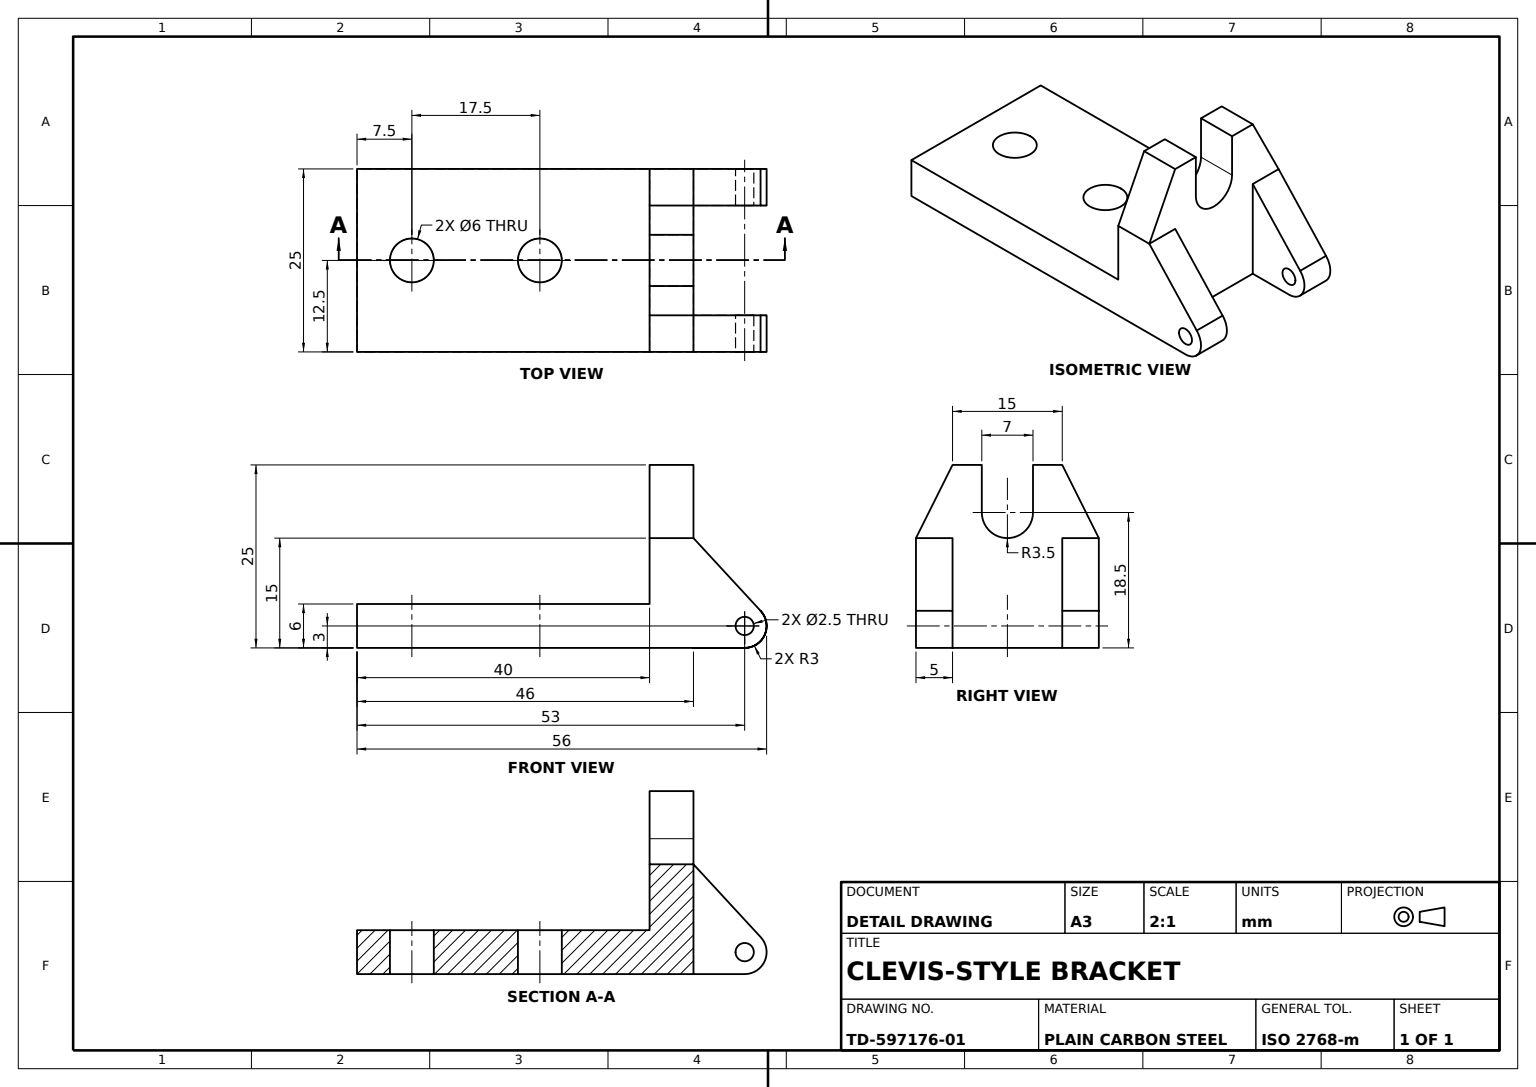
SolidWorks part; units mm, degrees
material "Plain Carbon Steel"
ref_plane "Front Plane" through (0, 0, 0) normal (0, 0, 1) x (1, 0, 0)
ref_plane "Top Plane" through (0, 0, 0) normal (0, 1, 0) x (1, 0, 0)
ref_plane "Right Plane" through (0, 0, 0) normal (1, 0, 0) x (0, 0, -1)
sketch "Base Profile Sketch" plane through (0, 0, 0) normal (0, 0, 1) x (1, 0, 0)
  line L0 (0, 0) -> (40, 0)
  line L1 (0, 0) -> (0, 6)
  line L2 (0, 6) -> (40, 6)
  line L3 (40, 6) -> (40, 0)
  dimension "D1" = 40
  dimension "D2" = 6
extrude "Base Body" add sketch "Base Profile Sketch" along normal blind 25
sketch "Upright Block Sketch" plane through (0, 0, 25) normal (0, 0, 1) x (1, 0, 0)
  line L0 (40, 0) -> (46, 0)
  line L1 (46, 0) -> (46, 15)
  line L2 (46, 15) -> (40, 15)
  line L3 (40, 15) -> (40, 0)
  line L4 (0, 6) -> (0, 0) construction
  line L5 (0, 0) -> (40, 0) construction
  dimension "D1" = 46
  dimension "D2" = 15
extrude "Upright Block" add sketch "Upright Block Sketch" against normal blind 25
sketch "Clevis Slot Profile Sketch" plane through (40, 0, 0) normal (-1, 0, 0) x (0, 0, 1)
  line L1 (25, 6) -> (0, 6) construction
  line L3 (9, 18.5) -> (9, 25)
  line L4 (16, 18.5) -> (16, 25)
  line L5 (16, 25) -> (20, 25)
  line L6 (20, 25) -> (25, 15)
  line L7 (9, 25) -> (5, 25)
  line L8 (5, 25) -> (0, 15)
  line L12 (0, 6) -> (25, 6)
  line L13 (25, 6) -> (25, 15)
  line L14 (25, 15) -> (0, 15)
  line L15 (0, 15) -> (0, 6)
  line L18 (25, 15) -> (0, 15)
  arc A0 (9, 18.5) -> (16, 18.5) centre (12.5, 18.5) ccw
  line M7 (25, 15) -> (0, 15)
  dimension "D1" = 0
  dimension "D2" = 3.5
  dimension "D3" = 5
  dimension "D4" = 19
extrude "Slotted Clevis Plate" add sketch "Clevis Slot Profile Sketch" against normal blind 6 contours A0 L6 L5 L4 M7 | A0 L3 L7 L8 L18
sketch "Lug 1 Sketch" plane through (0, 0, 25) normal (0, 0, 1) x (1, 0, 0)
  line L0 (46, 0) -> (53, 0)
  line L1 (0, 6) -> (0, 0) construction
  line L2 (46, 0) -> (46, 15)
  line L3 (46, 0) -> (46, 15) construction
  line L4 (46, 15) -> (55.171, 5.0704)
  line L5 (0, 0) -> (46, 0) construction
  arc A0 (53, 0) -> (55.171, 5.0704) centre (53, 3) ccw
  dimension "D1" = 3
  dimension "D2" = 53
  dimension "D3" = 55.171
  dimension "D4" = 15
extrude "Lug 1" add sketch "Lug 1 Sketch" against normal blind 5
sketch "Lug 1 Pin Hole Sketch" plane through (0, 0, 25) normal (0, 0, 1) x (1, 0, 0)
  circle A0 centre (53, 3) radius 1.25
  dimension "D1" = 2.5
  dimension "D2" = 2.5
extrude "Lug 1 Pin Hole" cut sketch "Lug 1 Pin Hole Sketch" against normal blind 5
sketch "Lug 2 Sketch" plane through (0, 0, 0) normal (0, 0, -1) x (-1, 0, 0)
  line L0 (-46, 0) -> (-53, 0)
  line L1 (-46, 15) -> (-55.171, 5.0704)
  line L2 (-46, 15) -> (-46, 0)
  arc A0 (-55.171, 5.0704) -> (-53, 0) centre (-53, 3) ccw
  dimension "D1" = 6
extrude "Lug 2" add sketch "Lug 2 Sketch" against normal blind 5
sketch "Lug 2 Pin Hole Sketch" plane through (0, 0, 0) normal (0, 0, -1) x (-1, 0, 0)
  circle A0 centre (-53, 3) radius 1.25
  dimension "D1" = 2.5
  dimension "D2" = 2.5
extrude "Lug 2 Pin Hole" cut sketch "Lug 2 Pin Hole Sketch" against normal blind 5
sketch "Mounting Holes Sketch" plane through (0, 6, 0) normal (0, 1, 0) x (1, 0, 0)
  line L0 (0, -25) -> (0, 0) construction
  line L1 (40, 0) -> (0, 0) construction
  circle A0 centre (7.5, -12.5) radius 3
  circle A1 centre (25, -12.5) radius 3
  dimension "D1" = 6
  dimension "D2" = 6
  dimension "D5" = 6
  dimension "D3" = 7.5
  dimension "D4" = 17.5
  dimension "D6" = 12.5
extrude "Mounting Holes 2xØ6" cut sketch "Mounting Holes Sketch" against normal blind 6
